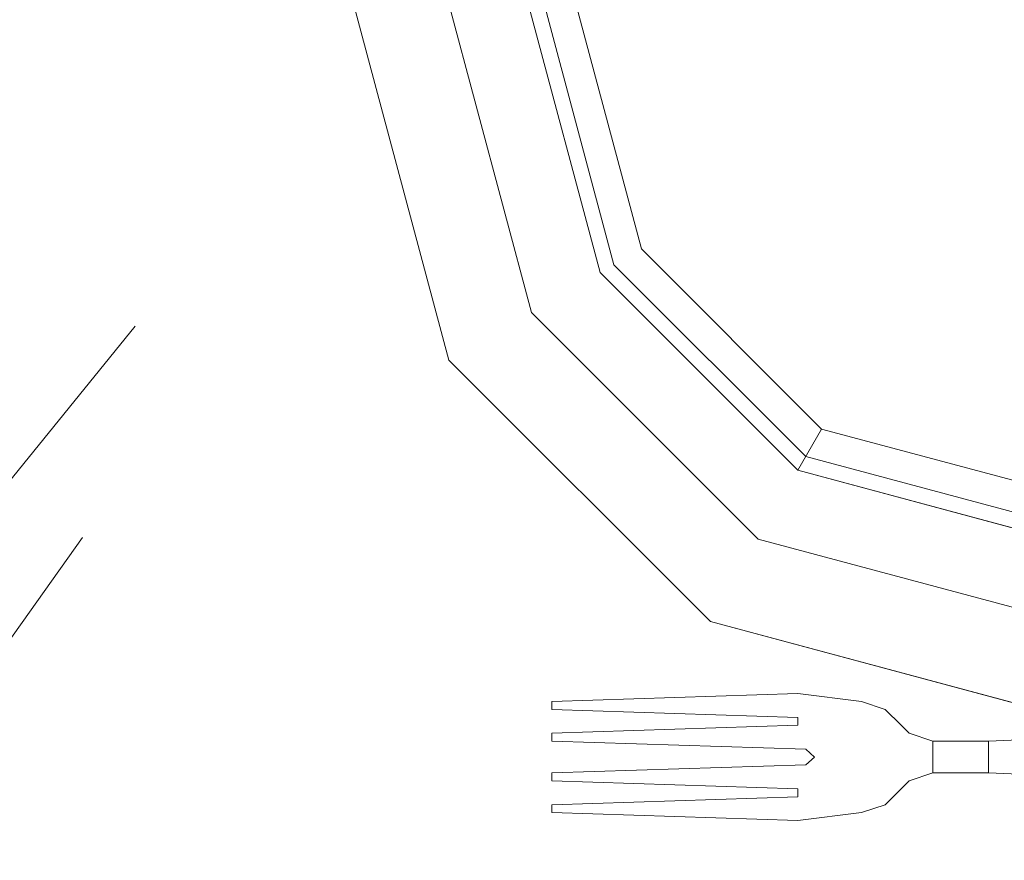
# Model space of a CAD drawing. Units: inches. Extents: x 375 to 1122, y 27 to 1069.
# Tile 28 of 155: x 731.646 to 739.279, y 270.593 to 277.109. Entities that reach past the tile are written whole.
import ezdxf

# ---------------------------------------------------------------- set-up
doc = ezdxf.new("R2010")
doc.units = ezdxf.units.IN
doc.layers.add('A-ANNO-DIMS', color=2, linetype='Continuous', lineweight=18)
doc.layers.add('Furniture', color=30, linetype='Continuous', lineweight=18)
doc.styles.get("Standard").update_dxf_attribs({"font": 'arial.ttf'})
doc.dimstyles.new('ISO-25', dxfattribs={"dimtxt": 12, "dimasz": 2.5, "dimexe": 1.5, "dimexo": 1.5, "dimtad": 1, "dimdec": 1, "dimlunit": 3, "dimtxsty": 'Standard', "dimblk": 'ARCHTICK', "dimcen": 2.5, "dimadec": 0, "dimazin": 0, "dimtfac": 1, "dimtdec": 1, "dimtmove": 0, "dimatfit": 3, "dimfxl": 1.5, "dimfxlon": 1, "dimarcsym": 0})

# ---------------------------------------------------------------- blocks, each defined once
blk = doc.blocks.new('A$C403C54AD')
for p, q in [((1.88351, 1.33067, -0.03581), (1.88197, 1.33529, -0.03534)), ((1.88351, 1.33067, -0.03888), (1.88197, 1.33529, -0.03842)), ((1.78922, 1.18993, 0.03663), (1.95298, 1.05694, 0.03663)), ((1.83016, 1.1797, 0.03663), (1.90181, 1.12855, 0.03663))]:
    blk.add_line(p, q)
for points, invisible_edges in [([(1.86812, 1.3907, -0.03153), (1.87735, 1.3907, -0.03153), (1.87581, 1.3553, -0.02863), (1.86966, 1.3553, -0.02863)], 1), ([(1.86812, 1.3907, -0.03153), (1.86812, 1.3907, -0.03461), (1.86966, 1.3553, -0.03122), (1.86966, 1.3553, -0.02863)], 5), ([(1.86812, 1.3907, -0.03461), (1.87735, 1.3907, -0.03461), (1.87581, 1.3553, -0.03122), (1.86966, 1.3553, -0.03122)], 1), ([(1.87581, 1.3553, -0.02863), (1.87581, 1.3553, -0.03122), (1.87735, 1.3907, -0.03461), (1.87735, 1.3907, -0.03153)], 5), ([(1.86966, 1.3553, -0.03122), (1.86966, 1.3553, -0.02863), (1.86966, 1.34452, -0.03071), (1.86966, 1.34452, -0.0333)], 5), ([(1.87581, 1.34452, -0.0333), (1.87581, 1.34452, -0.03071), (1.87581, 1.3553, -0.02863), (1.87581, 1.3553, -0.03122)], 5), ([(1.86966, 1.34452, -0.03071), (1.87581, 1.34452, -0.03071), (1.87735, 1.33991, -0.03306), (1.86812, 1.33991, -0.03306)], 4), ([(1.86966, 1.34452, -0.03071), (1.86966, 1.34452, -0.0333), (1.86812, 1.33991, -0.03584), (1.86812, 1.33991, -0.03306)], 5), ([(1.86966, 1.34452, -0.0333), (1.87581, 1.34452, -0.0333), (1.87735, 1.33991, -0.03584), (1.86812, 1.33991, -0.03584)], 4), ([(1.87581, 1.34452, -0.0333), (1.87581, 1.34452, -0.03071), (1.87735, 1.33991, -0.03306), (1.87735, 1.33991, -0.03584)], 5), ([(1.87735, 1.33991, -0.03306), (1.86812, 1.33991, -0.03306), (1.86658, 1.33837, -0.0341), (1.87889, 1.33837, -0.0341)], 5), ([(1.87735, 1.33991, -0.03584), (1.86812, 1.33991, -0.03584), (1.86658, 1.33837, -0.03718), (1.87889, 1.33837, -0.03718)], 5), ([(1.86812, 1.33991, -0.03584), (1.86812, 1.33991, -0.03306), (1.86658, 1.33837, -0.0341), (1.86658, 1.33837, -0.03718)], 1), ([(1.87735, 1.33991, -0.03306), (1.87735, 1.33991, -0.03584), (1.87889, 1.33837, -0.03718), (1.87889, 1.33837, -0.0341)], 1), ([(1.87889, 1.33837, -0.03718), (1.86658, 1.33837, -0.03718), (1.8635, 1.33529, -0.03842), (1.88197, 1.33529, -0.03842)], 5), ([(1.87889, 1.33837, -0.0341), (1.86658, 1.33837, -0.0341), (1.8635, 1.33529, -0.03534), (1.88197, 1.33529, -0.03534)], 5), ([(1.8635, 1.33529, -0.03534), (1.88197, 1.33529, -0.03534), (1.88351, 1.33067, -0.03581), (1.86196, 1.33067, -0.03581)], 5), ([(1.8635, 1.33529, -0.03842), (1.88197, 1.33529, -0.03842), (1.88351, 1.33067, -0.03888), (1.86196, 1.33067, -0.03888)], 5), ([(1.8635, 1.33529, -0.03842), (1.8635, 1.33529, -0.03534), (1.86196, 1.33067, -0.03581), (1.86196, 1.33067, -0.03888)], 4), ([(1.88197, 1.33529, -0.03534), (1.88197, 1.33529, -0.03842), (1.88351, 1.33067, -0.03888), (1.88351, 1.33067, -0.03581)], 4), ([(1.86196, 1.33067, -0.03581), (1.86658, 1.31836, -0.03521), (1.86504, 1.31836, -0.03521), (1.86042, 1.31836, -0.03521)], 5), ([(1.86196, 1.33067, -0.03888), (1.86658, 1.31836, -0.03829), (1.86504, 1.31836, -0.03829), (1.86042, 1.31836, -0.03829)], 5), ([(1.86196, 1.33067, -0.03581), (1.86196, 1.33067, -0.03888), (1.86042, 1.31836, -0.03829), (1.86042, 1.31836, -0.03521)], 1), ([(1.86196, 1.33067, -0.03581), (1.87273, 1.32156, -0.0356), (1.8712, 1.3199, -0.03545), (1.86658, 1.31836, -0.03521)], 13), ([(1.86196, 1.33067, -0.03581), (1.87273, 1.32156, -0.0356), (1.88351, 1.33067, -0.03581), (1.86196, 1.33067, -0.03581)], 7), ([(1.86196, 1.33067, -0.03888), (1.87273, 1.32156, -0.03868), (1.88351, 1.33067, -0.03888), (1.86196, 1.33067, -0.03888)], 7), ([(1.86196, 1.33067, -0.03888), (1.87273, 1.32156, -0.03868), (1.8712, 1.3199, -0.03853), (1.86658, 1.31836, -0.03829)], 13), ([(1.88351, 1.33067, -0.03581), (1.87273, 1.32156, -0.0356), (1.87427, 1.3199, -0.03545), (1.87889, 1.31836, -0.03521)], 13), ([(1.88351, 1.33067, -0.03888), (1.87273, 1.32156, -0.03868), (1.87427, 1.3199, -0.03853), (1.87889, 1.31836, -0.03829)], 13), ([(1.88351, 1.33067, -0.03581), (1.87889, 1.31836, -0.03521), (1.88043, 1.31836, -0.03521), (1.88505, 1.31836, -0.03521)], 5), ([(1.88351, 1.33067, -0.03888), (1.87889, 1.31836, -0.03829), (1.88043, 1.31836, -0.03829), (1.88505, 1.31836, -0.03829)], 5), ([(1.88351, 1.33067, -0.03888), (1.88351, 1.33067, -0.03581), (1.88505, 1.31836, -0.03521), (1.88505, 1.31836, -0.03829)], 1), ([(1.86658, 1.31836, -0.03521), (1.8712, 1.3199, -0.03545), (1.86966, 1.27064, -0.02811), (1.86812, 1.27064, -0.02811)], 1), ([(1.86658, 1.31836, -0.03829), (1.8712, 1.3199, -0.03853), (1.86966, 1.27064, -0.03119), (1.86812, 1.27064, -0.03119)], 1), ([(1.87427, 1.3199, -0.03545), (1.87889, 1.31836, -0.03521), (1.87735, 1.27064, -0.02811), (1.87581, 1.27064, -0.02811)], 1), ([(1.87427, 1.3199, -0.03853), (1.87889, 1.31836, -0.03829), (1.87735, 1.27064, -0.03119), (1.87581, 1.27064, -0.03119)], 1), ([(1.86504, 1.31836, -0.03521), (1.86042, 1.31836, -0.03521), (1.86196, 1.27064, -0.02811), (1.8635, 1.27064, -0.02811)], 1), ([(1.86504, 1.31836, -0.03829), (1.86042, 1.31836, -0.03829), (1.86196, 1.27064, -0.03119), (1.8635, 1.27064, -0.03119)], 1), ([(1.88043, 1.31836, -0.03521), (1.88505, 1.31836, -0.03521), (1.88351, 1.27064, -0.02811), (1.88197, 1.27064, -0.02811)], 1), ([(1.88043, 1.31836, -0.03829), (1.88505, 1.31836, -0.03829), (1.88351, 1.27064, -0.03119), (1.88197, 1.27064, -0.03119)], 1)]:
    blk.add_3dface(points, dxfattribs=dict(invisible_edges=invisible_edges))
at = {"linetype": 'ByBlock'}
for points, invisible_edges in [([(1.72651, 1.2691, -0.02965), (1.72651, 1.37069, -0.02965), (1.72651, 1.37069, -0.02965), (1.7773, 1.28271, -0.02965)], 5), ([(1.81449, 1.3199, -0.02965), (1.72651, 1.37069, -0.02965), (1.72651, 1.37069, -0.02965), (1.8281, 1.37069, -0.02965)], 5), ([(1.7773, 1.28271, -0.02965), (1.72651, 1.37069, -0.02965), (1.72651, 1.37069, -0.02965), (1.81449, 1.3199, -0.02965)], 5), ([(1.83048, 1.31066, -0.02349), (1.81449, 1.3199, -0.02965), (1.8281, 1.37069, -0.02965), (1.84657, 1.37069, -0.02349)], 5), ([(1.81715, 1.31836, -0.03734), (1.84648, 1.30143, -0.02811), (1.86504, 1.37069, -0.02811), (1.83118, 1.37069, -0.03734)], 5), ([(1.84648, 1.30143, -0.02349), (1.83048, 1.31066, -0.02349), (1.84657, 1.37069, -0.02349), (1.86504, 1.37069, -0.02349)], 5), ([(1.77423, 1.28804, -0.04658), (1.77884, 1.28005, -0.03734), (1.81715, 1.31836, -0.03734), (1.80916, 1.32297, -0.04658)], 1), ([(1.78654, 1.26672, -0.02349), (1.7773, 1.28271, -0.02965), (1.81449, 1.3199, -0.02965), (1.83048, 1.31066, -0.02349)], 5), ([(1.77884, 1.28005, -0.03734), (1.79578, 1.25072, -0.02811), (1.84648, 1.30143, -0.02811), (1.81715, 1.31836, -0.03734)], 5), ([(1.79578, 1.25072, -0.02349), (1.78654, 1.26672, -0.02349), (1.83048, 1.31066, -0.02349), (1.84648, 1.30143, -0.02349)], 5), ([(1.72651, 1.27526, -0.04658), (1.72651, 1.26602, -0.03734), (1.77884, 1.28005, -0.03734), (1.77423, 1.28804, -0.04658)], 5), ([(1.72651, 1.25063, -0.02349), (1.72651, 1.2691, -0.02965), (1.7773, 1.28271, -0.02965), (1.78654, 1.26672, -0.02349)], 5), ([(1.72651, 1.26602, -0.03734), (1.72651, 1.23216, -0.02811), (1.79578, 1.25072, -0.02811), (1.77884, 1.28005, -0.03734)], 5), ([(1.72651, 1.23216, -0.02349), (1.72651, 1.25063, -0.02349), (1.78654, 1.26672, -0.02349), (1.79578, 1.25072, -0.02349)], 5)]:
    blk.add_3dface(points, dxfattribs=dict(at, invisible_edges=invisible_edges))
for points in [[(1.80916, 1.32297, -0.04658), (1.81715, 1.31836, -0.03734), (1.83118, 1.37069, -0.03734), (1.82194, 1.37069, -0.04658)], [(1.84648, 1.30143, -0.02811), (1.84648, 1.30143, -0.02349), (1.86504, 1.37069, -0.02349), (1.86504, 1.37069, -0.02811)], [(1.79578, 1.25072, -0.02811), (1.79578, 1.25072, -0.02349), (1.84648, 1.30143, -0.02349), (1.84648, 1.30143, -0.02811)], [(1.72651, 1.23216, -0.02811), (1.72651, 1.23216, -0.02349), (1.79578, 1.25072, -0.02349), (1.79578, 1.25072, -0.02811)]]:
    blk.add_3dface(points, dxfattribs=at)
for points in [[(1.87581, 1.3553, -0.02863), (1.86966, 1.3553, -0.02863), (1.86966, 1.34452, -0.03071), (1.87581, 1.34452, -0.03071)], [(1.87581, 1.3553, -0.03122), (1.86966, 1.3553, -0.03122), (1.86966, 1.34452, -0.0333), (1.87581, 1.34452, -0.0333)], [(1.86658, 1.33837, -0.0341), (1.86658, 1.33837, -0.03718), (1.8635, 1.33529, -0.03842), (1.8635, 1.33529, -0.03534)], [(1.87889, 1.33837, -0.03718), (1.87889, 1.33837, -0.0341), (1.88197, 1.33529, -0.03534), (1.88197, 1.33529, -0.03842)], [(1.87273, 1.32156, -0.03868), (1.87273, 1.32156, -0.0356), (1.8712, 1.3199, -0.03545), (1.8712, 1.3199, -0.03853)], [(1.87427, 1.3199, -0.03545), (1.87427, 1.3199, -0.03853), (1.87273, 1.32156, -0.03868), (1.87273, 1.32156, -0.0356)], [(1.86966, 1.27064, -0.03119), (1.86966, 1.27064, -0.02811), (1.8712, 1.3199, -0.03545), (1.8712, 1.3199, -0.03853)], [(1.87427, 1.3199, -0.03853), (1.87427, 1.3199, -0.03545), (1.87581, 1.27064, -0.02811), (1.87581, 1.27064, -0.03119)], [(1.86042, 1.31836, -0.03829), (1.86042, 1.31836, -0.03521), (1.86196, 1.27064, -0.02811), (1.86196, 1.27064, -0.03119)], [(1.8635, 1.27064, -0.02811), (1.8635, 1.27064, -0.03119), (1.86504, 1.31836, -0.03829), (1.86504, 1.31836, -0.03521)], [(1.86658, 1.31836, -0.03829), (1.86658, 1.31836, -0.03521), (1.86504, 1.31836, -0.03521), (1.86504, 1.31836, -0.03829)], [(1.86658, 1.31836, -0.03829), (1.86658, 1.31836, -0.03521), (1.86812, 1.27064, -0.02811), (1.86812, 1.27064, -0.03119)], [(1.87735, 1.27064, -0.02811), (1.87735, 1.27064, -0.03119), (1.87889, 1.31836, -0.03829), (1.87889, 1.31836, -0.03521)], [(1.88043, 1.31836, -0.03521), (1.88043, 1.31836, -0.03829), (1.87889, 1.31836, -0.03829), (1.87889, 1.31836, -0.03521)], [(1.88043, 1.31836, -0.03521), (1.88043, 1.31836, -0.03829), (1.88197, 1.27064, -0.03119), (1.88197, 1.27064, -0.02811)], [(1.88351, 1.27064, -0.02811), (1.88351, 1.27064, -0.03119), (1.88505, 1.31836, -0.03829), (1.88505, 1.31836, -0.03521)], [(1.86196, 1.27064, -0.03119), (1.86196, 1.27064, -0.02811), (1.8635, 1.27064, -0.02811), (1.8635, 1.27064, -0.03119)], [(1.86812, 1.27064, -0.03119), (1.86812, 1.27064, -0.02811), (1.86966, 1.27064, -0.02811), (1.86966, 1.27064, -0.03119)], [(1.87581, 1.27064, -0.03119), (1.87581, 1.27064, -0.02811), (1.87735, 1.27064, -0.02811), (1.87735, 1.27064, -0.03119)], [(1.88197, 1.27064, -0.03119), (1.88197, 1.27064, -0.02811), (1.88351, 1.27064, -0.02811), (1.88351, 1.27064, -0.03119)]]:
    blk.add_3dface(points)
blk = doc.blocks.new('_ArchTick')
at = {"color": 0, "linetype": 'ByBlock', "const_width": 0.15}
blk.add_lwpolyline([(-0.5, -0.5), (0.5, 0.5)], dxfattribs=at)
blk = doc.blocks.new('*D94')
at = {"layer": 'A-ANNO-DIMS', "color": 0, "lineweight": -2, "transparency": 16777216}
for p, q in [((734.0073, 117.5277), (734.0073, 114.5277)), ((773.0073, 117.5277), (773.0073, 114.5277)), ((734.0073, 116.0277), (773.0073, 116.0277))]:
    blk.add_line(p, q, dxfattribs=at)
at = {"layer": 'Defpoints', "color": 0, "transparency": 16777216}
for p in [(734.0073, 667.5277), (773.0073, 667.5277), (773.0073, 116.0277)]:
    blk.add_point(p, dxfattribs=at)
at = {"layer": 'A-ANNO-DIMS', "color": 0, "lineweight": -2, "transparency": 16777216, "xscale": 2.5, "yscale": 2.5, "zscale": 2.5, "rotation": 180}
blk.add_blockref('_ArchTick', (734.0073, 116.0277), dxfattribs=at)
at = {"layer": 'A-ANNO-DIMS', "color": 0, "lineweight": -2, "transparency": 16777216, "xscale": 2.5, "yscale": 2.5, "zscale": 2.5}
blk.add_blockref('_ArchTick', (773.0073, 116.0277), dxfattribs=at)
at = {"layer": 'A-ANNO-DIMS', "color": 0, "transparency": 16777216, "insert": (753.5073, 122.7837), "char_height": 12, "attachment_point": 5}
blk.add_mtext('3\'-3"', dxfattribs=at)

msp = doc.modelspace()

# ---------------------------------------------------------------- block references
at = {"layer": 'Furniture', "xscale": 39.9918517141215, "yscale": 39.9918517141215, "zscale": 39.9918517141215, "rotation": 270}
msp.add_blockref('A$C403C54AD', (684.9549, 346.2875, 0.024), dxfattribs=at)

# ---------------------------------------------------------------- dimensions: what is measured, and where the dimension line sits
at = {"layer": 'A-ANNO-DIMS'}
dim = msp.add_linear_dim(base=(773.0073, 116.0277), p1=(734.0073, 667.5277), p2=(773.0073, 667.5277), dimstyle='ISO-25', override={"dimdec": 1, "dimlfac": 1, "dimrnd": 0, "dimzin": 1, "dimdsep": 46, "dimlunit": 4, "dimfrac": 2}, dxfattribs=at)
dim.commit()
dim.dimension.update_dxf_attribs({"geometry": '*D94', "text_midpoint": (753.5073, 122.7837)})

doc.saveas('drawing.dxf')
